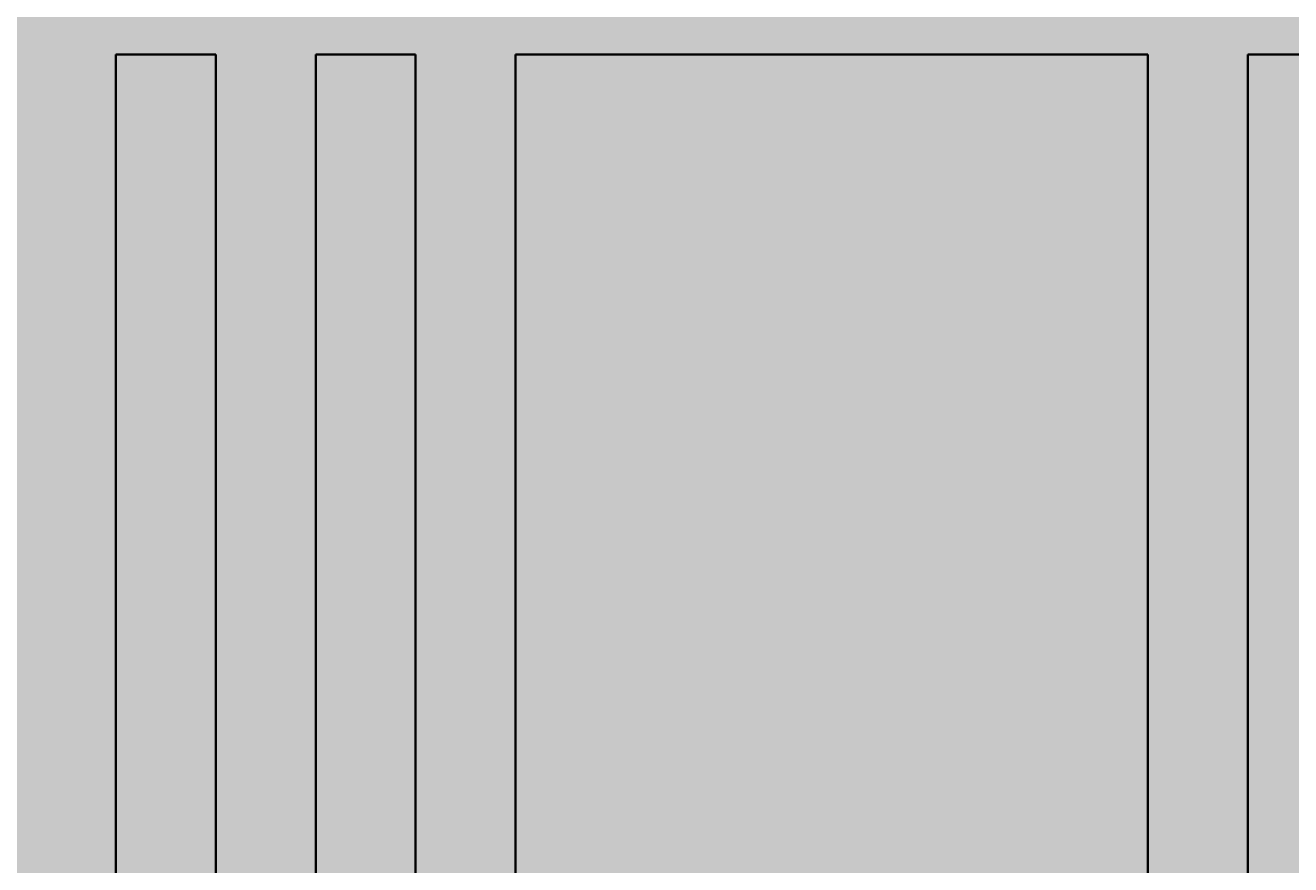
# Model space of a CAD drawing. Units: inches. Extents: x -1 to 292, y -3 to 199.
# Tile 21 of 52: x 68 to 106, y 68 to 93. Entities that reach past the tile are written whole.
import ezdxf

# ---------------------------------------------------------------- set-up
doc = ezdxf.new("R2010")
doc.units = ezdxf.units.IN
doc.header["$MEASUREMENT"] = 0
for name, color, linetype, lineweight in [('M-DIMS', 2, 'Continuous', 18), ('M-EQPM', 7, 'Continuous', 35), ('M-PATT', 8, 'Continuous', 13)]:
    doc.layers.add(name, color=color, linetype=linetype, lineweight=lineweight)
doc.styles.get("Standard").update_dxf_attribs({"font": 'arial.ttf'})
doc.dimstyles.get("Standard").update_dxf_attribs({"dimtxt": 0.18, "dimasz": 0.18, "dimexe": 0.18, "dimexo": 0.0625, "dimgap": 0.09, "dimtad": 0, "dimtih": 1, "dimtoh": 1, "dimdec": 4, "dimzin": 0, "dimdsep": 46, "dimtxsty": 'Standard', "dimcen": 0.09, "dimadec": 0, "dimazin": 0, "dimtfac": 1, "dimtdec": 4, "dimtofl": 0, "dimtmove": 0, "dimatfit": 3, "dimfxl": 1, "dimtolj": 1, "dimtzin": 0, "dimarcsym": 0})

# ---------------------------------------------------------------- blocks, each defined once
blk = doc.blocks.new('BOILER-TUBE')
for p, q in [((0, 40.63), (0, 0)), ((3, 40.63), (3, 0))]:
    blk.add_line(p, q)
for points in [[(0, 40.63), (3, 40.63)], [(3, 0), (0, 0)]]:
    blk.add_lwpolyline(points)
blk = doc.blocks.new('*D8')
at = {"layer": 'Defpoints', "color": 0, "transparency": 16777216}
for p in [(-0.662, 126.765), (111.488, 126.765), (69.013, 25.514)]:
    blk.add_point(p, dxfattribs=at)
at = {"layer": 'M-DIMS', "color": 0, "lineweight": -2, "transparency": 16777216}
for p, q in [((111.426, 126.765), (-0.842, 126.765)), ((-0.662, 126.585), (-0.662, 76.321)), ((-0.662, 25.694), (-0.662, 75.958)), ((68.951, 25.514), (-0.842, 25.514))]:
    blk.add_line(p, q, dxfattribs=at)
at = {"layer": 'M-DIMS', "color": 0, "transparency": 16777216}
for points in [[(-0.692, 126.585), (-0.632, 126.585), (-0.662, 126.765)], [(-0.692, 25.694), (-0.632, 25.694), (-0.662, 25.514)]]:
    blk.add_solid(points, dxfattribs=at)
at = {"layer": 'M-DIMS', "color": 0, "transparency": 16777216, "insert": (-0.662, 76.14), "char_height": 0.18, "attachment_point": 5}
blk.add_mtext('\\A1;101.25', dxfattribs=at)

msp = doc.modelspace()

# ---------------------------------------------------------------- hatches: boundary and pattern name
at = {"layer": 'M-PATT'}
h = msp.add_hatch(color=256, dxfattribs=at)
h.set_gradient(color1=(237, 31, 36), color2=(242, 113, 114), tint=1, name='CYLINDER')
h.paths.add_polyline_path([(106.0735, 105.9941), (106.0735, 106.9941), (108.0603, 106.9941), (107.8488, 107.6501), (57.8007, 107.6501, 0.4142136), (49.9241, 99.7735), (52.3176, 101.3278), (55.0097, 99.7735), (57.4032, 101.3278), (60.0953, 99.7735), (62.4888, 101.3278), (65.1809, 99.7735), (67.5744, 101.3278), (70.2665, 99.7735), (72.66, 101.3278), (75.3521, 99.7735), (77.7456, 101.3278), (80.4377, 99.7735), (82.8312, 101.3278), (85.5233, 99.7735), (87.9168, 101.3278), (90.6089, 99.7735), (93.0024, 101.3278), (95.6945, 99.7735), (98.088, 101.3278), (100.7801, 99.7735), (103.1736, 101.3278), (105.8657, 99.7735), (108.2592, 101.3278), (110.9513, 99.7735), (113.3448, 101.3278), (116.0369, 99.7735), (118.4304, 101.3278), (121.1225, 99.7735), (123.516, 101.3278), (126.2082, 99.7735), (128.6016, 101.3278), (131.2938, 99.7735), (133.6872, 101.3278), (136.3794, 99.7735), (138.7728, 101.3278), (141.465, 99.7735), (143.8584, 101.3278), (146.5506, 99.7735), (148.944, 101.3278), (151.6362, 99.7735), (154.0296, 101.3278), (156.7218, 99.7735), (159.1152, 101.3278), (160.6222, 100.4578), (160.6222, 107.6501), (115.4883, 107.6501), (115.4883, 106.9941), (120.9032, 106.9941), (120.9032, 105.9941), (120.9032, 103.3981), (106.0735, 103.3981)])
h.paths.add_polyline_path([(169.176, 107.6501), (162.1623, 107.6501), (162.1623, 100.004), (164.2008, 101.3278), (166.893, 99.7735), (169.2864, 101.3278), (171.9786, 99.7735), (174.372, 101.3278), (177.0526, 99.7802, 0.4139642)])
h.paths.add_polyline_path([(111.4883, 107.6501), (107.8488, 107.6501), (108.0603, 106.9941), (111.4883, 106.9941)], flags=17)
h.paths.add_polyline_path([(61.6788, 91.897), (57.8007, 91.897, -0.1099266), (54.4604, 92.6403), (43.2011, 92.6403), (23.9502, 84.4688), (23.9502, 58.376), (43.2011, 47.2615), (50.9409, 47.2615, -0.2705926), (57.8007, 51.2672), (61.6788, 51.2672)])
h.paths.add_polyline_path([(73.6788, 91.897), (70.6788, 91.897), (70.6788, 51.2672), (73.6788, 51.2672)])
h.paths.add_polyline_path([(79.6788, 91.897), (76.6788, 91.897), (76.6788, 51.2672), (79.6788, 51.2672)])
h.paths.add_polyline_path([(67.6788, 91.897), (64.6788, 91.897), (64.6788, 51.2672), (67.6788, 51.2672)])
h.paths.add_polyline_path([(101.6788, 91.897), (82.6788, 91.897), (82.6788, 51.2672), (101.6788, 51.2672)])
h.paths.add_polyline_path([(107.6788, 91.897), (104.6788, 91.897), (104.6788, 51.2672), (107.6788, 51.2672)])
h.paths.add_polyline_path([(113.6788, 91.897), (110.6788, 91.897), (110.6788, 51.2672), (113.6788, 51.2672)])
h.paths.add_polyline_path([(119.6788, 91.897), (116.6788, 91.897), (116.6788, 51.2672), (119.6788, 51.2672)])
h.paths.add_polyline_path([(141.6788, 91.897), (122.6788, 91.897), (122.6788, 51.2672), (141.6788, 51.2672)])
h.paths.add_polyline_path([(147.6788, 91.897), (144.6788, 91.897), (144.6788, 51.2672), (147.6788, 51.2672)])
h.paths.add_polyline_path([(153.6788, 91.897), (150.6788, 91.897), (150.6788, 51.2672), (153.6788, 51.2672)])
h.paths.add_polyline_path([(159.6788, 91.897), (156.6788, 91.897), (156.6788, 51.2672), (159.6788, 51.2672)])
h.paths.add_polyline_path([(179.5897, 92.6403), (172.5163, 92.6403, -0.1099266), (169.176, 91.897), (162.6788, 91.897), (162.6788, 51.2672), (169.176, 51.2672, -0.2705926), (176.0358, 47.2615), (179.5897, 47.2615)])
h.paths.add_polyline_path([(203.0265, 84.4688), (183.7755, 92.6403), (181.5897, 92.6403), (181.5897, 47.2615), (183.7755, 47.2615), (203.0265, 58.376)])
h.paths.add_polyline_path([(184.4188, 61.52), (200.7224, 61.52), (200.7224, 77.7532), (184.4188, 77.7532)], flags=24)
h = msp.add_hatch(color=256, dxfattribs=at)
h.set_gradient(color1=(0, 255, 255), color2=(0, 255, 255), tint=1)
h.paths.add_polyline_path([(75.3521, 99.7735), (72.66, 101.3278), (70.2665, 99.7735), (67.5744, 101.3278), (65.1809, 99.7735), (62.4888, 101.3278), (60.0953, 99.7735), (57.4032, 101.3278), (55.0097, 99.7735), (52.3176, 101.3278), (49.9241, 99.7735, 0.4142136), (57.8007, 91.897), (61.6788, 91.897), (61.6788, 51.2672), (57.8007, 51.2672, 0.8088808), (54.5813, 36.2021), (65.0947, 51.2672), (64.6788, 51.2672), (64.6788, 91.897), (67.6788, 91.897), (67.6788, 51.2672), (65.0947, 51.2672), (54.5813, 36.2021, 0.1056561), (57.8007, 35.5141), (169.176, 35.5141, 1), (169.176, 51.2672), (162.6788, 51.2672), (162.6788, 91.897), (169.176, 91.897, 0.4144629), (177.0526, 99.7802), (174.372, 101.3278), (171.9786, 99.7735), (169.2864, 101.3278), (166.893, 99.7735), (164.2008, 101.3278), (162.1623, 100.004), (162.1623, 96.1027), (160.6222, 96.1027), (160.6222, 100.4578), (159.1152, 101.3278), (156.7218, 99.7735), (154.0296, 101.3278), (151.6362, 99.7735), (148.944, 101.3278), (146.5506, 99.7735), (143.8584, 101.3278), (141.465, 99.7735), (138.7728, 101.3278), (136.3794, 99.7735), (133.6872, 101.3278), (131.2938, 99.7735), (128.6016, 101.3278), (126.2082, 99.7735), (123.516, 101.3278), (121.1225, 99.7735), (118.4304, 101.3278), (116.0369, 99.7735), (113.3448, 101.3278), (110.9513, 99.7735), (108.2592, 101.3278), (105.8657, 99.7735), (103.1736, 101.3278), (100.7801, 99.7735), (98.088, 101.3278), (95.6945, 99.7735), (93.0024, 101.3278), (90.6089, 99.7735), (87.9168, 101.3278), (85.5233, 99.7735), (82.8312, 101.3278), (80.4377, 99.7735), (77.7456, 101.3278)])
h.paths.add_polyline_path([(79.6788, 91.897), (79.6788, 51.2672), (76.6788, 51.2672), (76.6788, 91.897)], flags=16)
h.paths.add_polyline_path([(73.6788, 91.897), (73.6788, 51.2672), (70.6788, 51.2672), (70.6788, 91.897)], flags=16)
h.paths.add_polyline_path([(82.6788, 91.897), (101.6788, 91.897), (101.6788, 51.2672), (82.6788, 51.2672)], flags=16)
h.paths.add_polyline_path([(104.6788, 91.897), (107.6788, 91.897), (107.6788, 51.2672), (104.6788, 51.2672)], flags=16)
h.paths.add_polyline_path([(110.6788, 91.897), (113.6788, 91.897), (113.6788, 51.2672), (110.6788, 51.2672)], flags=16)
h.paths.add_polyline_path([(116.6788, 91.897), (119.6788, 91.897), (119.6788, 51.2672), (116.6788, 51.2672)], flags=16)
h.paths.add_polyline_path([(122.6788, 91.897), (141.6788, 91.897), (141.6788, 51.2672), (144.6788, 51.2672), (144.6788, 91.897), (147.6788, 91.897), (147.6788, 51.2672), (122.6788, 51.2672)], flags=16)
h.paths.add_polyline_path([(150.6788, 91.897), (153.6788, 91.897), (153.6788, 51.2672), (150.6788, 51.2672)], flags=16)
h.paths.add_polyline_path([(156.6788, 91.897), (159.6788, 91.897), (159.6788, 51.2672), (156.6788, 51.2672)], flags=16)

# ---------------------------------------------------------------- linework, layer by layer
at = {"layer": 'M-EQPM'}
for p, q in [((82.6788, 91.897), (82.6788, 51.2672)), ((101.6788, 91.897), (101.6788, 51.2672))]:
    msp.add_line(p, q, dxfattribs=at)
msp.add_lwpolyline([(82.6788, 91.897), (101.6788, 91.897)], dxfattribs=at)

# ---------------------------------------------------------------- block references
for p in [(70.679, 51.267), (76.679, 51.267), (104.679, 51.267)]:
    msp.add_blockref('BOILER-TUBE', p, dxfattribs=at)

# ---------------------------------------------------------------- dimensions: what is measured, and where the dimension line sits
at = {"layer": 'M-DIMS'}
dim = msp.add_linear_dim(base=(-0.6625, 126.765), p1=(69.013, 25.5141), p2=(111.4883, 126.765), angle=90, dimstyle='Standard', override={"dimdec": 2, "dimlfac": 1, "dimrnd": 0, "dimzin": 0, "dimdsep": 46, "dimlunit": 2}, dxfattribs=at)
dim.commit()
dim.dimension.update_dxf_attribs({"geometry": '*D8', "text_midpoint": (-0.6625, 76.1396)})

doc.saveas('drawing.dxf')
